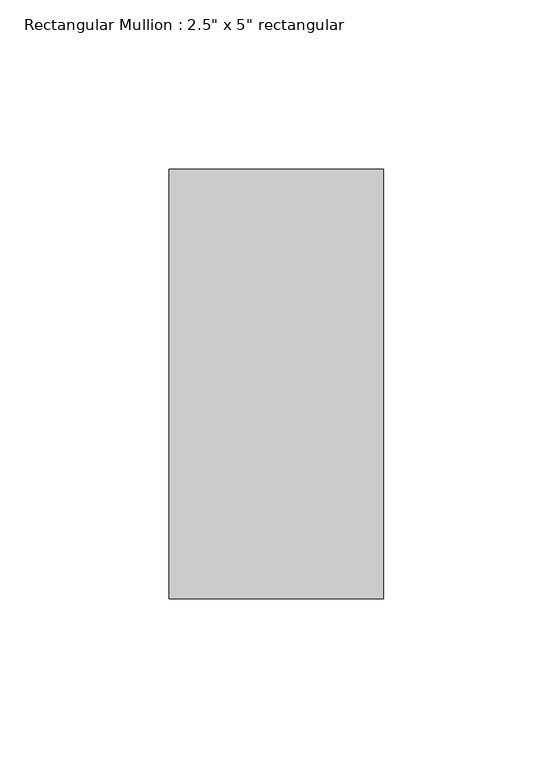
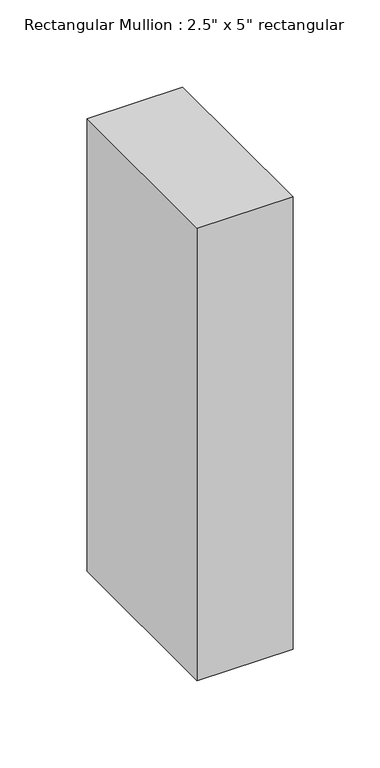
"""IFC4 building model written with IfcOpenShell, lengths in millimetres: member geometry."""

from ifc_helpers import new_model, si_unit, frame, origin, place, context, project, spatial, polyline, outline, extrude, source, transform, mapped, element, save


def member_3060f3e2(model_context):
    return source(origin(), model_context, "Body", "SweptSolid", [
        extrude(outline(polyline([(0.0, 63.5), (0.0, -63.5), (-63.5, -63.5), (-63.5, 63.5), (0.0, 63.5)])), frame((0.0, 0.0, -317.5), z_axis=(0.0, 0.0, 1.0), x_axis=(1.0, 0.0, 0.0)), (0.0, 0.0, 1.0), 317.5),
    ])


if __name__ == "__main__":
    model = new_model("IFC4")
    model_context = context("Model", 3, world=origin())
    ifc_project = project(units=[si_unit("LENGTHUNIT", "METRE", prefix="MILLI")], contexts=[model_context])
    site = spatial("IfcSite", under=ifc_project)
    building = spatial("IfcBuilding", under=site)
    placement = place(None, origin())
    member_shape = member_3060f3e2(model_context)
    element("IfcMember", 1, ObjectType="Rectangular Mullion : 2.5\" x 5\" rectangular", at=placement, inside=building, context=model_context, shape_type="MappedRepresentation", body=[
        mapped(member_shape, transform((0.0, 0.0, 0.0), x_axis=(1.0, 0.0, 0.0), y_axis=(0.0, 1.0, 0.0), z_axis=(0.0, 0.0, 1.0))),
    ])
    save(model, "model.ifc")

# Revit data of these elements
# Type "Rectangular Mullion : 2.5\" x 5\" rectangular"
#   built-in parameter 1007304 = 0.416667 (stored number, unit not read)
#   built-in parameter 1007301 = 0.104167 (stored number, unit not read)
#   built-in parameter 1007300 = 0.104167 (stored number, unit not read)
# Element 1 (IfcMember, "Rectangular Mullion : 2.5\" x 5\" rectangular")
#   Materials on its faces: "Aluminum"
# Materials
#   "Aluminum": class "Metal", colour RGB 247 247 247, transparency 0, Description = "Aluminum 6061", Cost = 0
